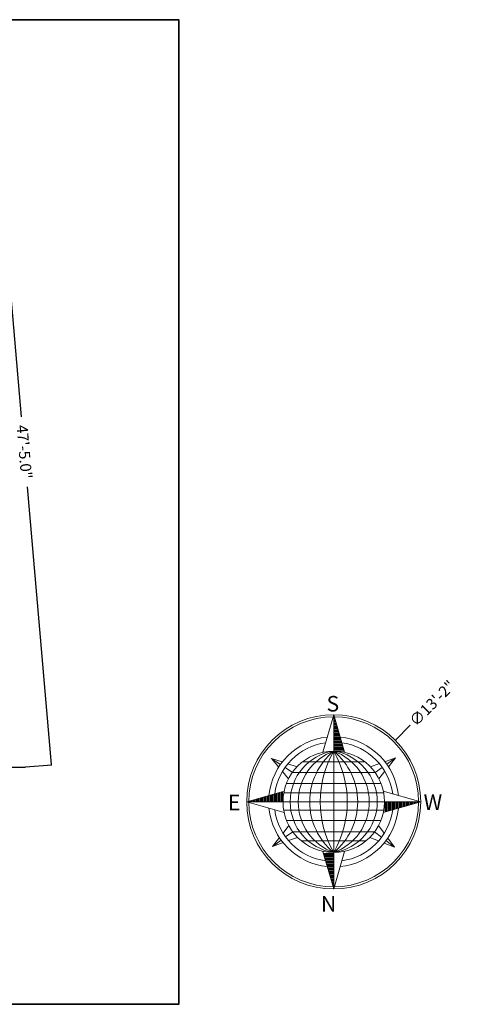
# Model space of a CAD drawing. Units: inches. Extents: x -269 to 4574, y -694 to 313.
# Tile 17 of 19: x 522 to 919, y -694 to 198. Entities that reach past the tile are written whole.
import ezdxf

# ---------------------------------------------------------------- set-up
doc = ezdxf.new("R2010")
doc.units = ezdxf.units.IN
doc.header["$MEASUREMENT"] = 0
for name, color, linetype, lineweight in [('A-ANNO-SYMB', 7, 'Continuous', 18), ('A-ANNO-SYMB-PATT', 7, 'Continuous', 13), ('BORDER', 7, 'Continuous', 35), ('C-PROP', 7, 'Continuous', 25), ('DIMENSION', 5, 'Continuous', 18)]:
    doc.layers.add(name, color=color, linetype=linetype, lineweight=lineweight)
doc.dimstyles.get("Standard").update_dxf_attribs({"dimtxt": 10, "dimasz": 0.18, "dimexe": 0.18, "dimexo": 0.0625, "dimgap": 0.09, "dimtad": 0, "dimdec": 1, "dimzin": 0, "dimdsep": 46, "dimlunit": 3, "dimtxsty": 'Standard', "dimcen": 0.09, "dimclrt": 7, "dimadec": 0, "dimazin": 0, "dimtfac": 1, "dimtdec": 1, "dimtofl": 0, "dimtmove": 0, "dimatfit": 3, "dimfxl": 1, "dimtolj": 1, "dimtzin": 0, "dimarcsym": 0})
pattern_1 = [(90, (-1638.3669, -937.0711), (-1, 0), [])]
pattern_2 = [(180, (-1638.3669, -937.0711), (-1e-16, -1), [])]

# ---------------------------------------------------------------- blocks, each defined once
blk = doc.blocks.new('*D35')
at = {"layer": 'Defpoints', "color": 0, "lineweight": 0, "transparency": 16777216}
for p in [(478.29, 88), (527.63, -478.86), (551.23, -476.8)]:
    blk.add_point(p, dxfattribs=at)
at = {"layer": 'DIMENSION', "color": 0, "lineweight": -2, "transparency": 16777216}
for p, q in [((478.36, 88.01), (502.07, 90.07)), ((501.91, 89.87), (523.81, -161.74)), ((551.21, -476.62), (529.31, -225.01)), ((527.69, -478.85), (551.41, -476.79))]:
    blk.add_line(p, q, dxfattribs=at)
at = {"layer": 'DIMENSION', "color": 0, "lineweight": 0, "transparency": 16777216}
for points in [[(501.94, 89.88), (501.88, 89.87), (501.89, 90.05)], [(551.24, -476.62), (551.18, -476.63), (551.23, -476.8)]]:
    blk.add_solid(points, dxfattribs=at)
at = {"layer": 'DIMENSION', "color": 0, "transparency": 16777216, "insert": (526.56, -193.38), "char_height": 10, "attachment_point": 5, "rotation": 274.97381}
blk.add_mtext('\\A1;47\'-5.0"', dxfattribs=at)
blk = doc.blocks.new('*D87')
at = {"layer": 'Defpoints', "color": 0, "lineweight": 0, "transparency": 16777216}
for p in [(862.88, -454.59), (751.27, -566.21)]:
    blk.add_point(p, dxfattribs=at)
at = {"layer": 'DIMENSION', "color": 0, "lineweight": -2, "transparency": 16777216}
for p, q in [((876.43, -441.04), (863, -454.47)), ((806.98, -510.4), (807.16, -510.4)), ((807.07, -510.49), (807.07, -510.31))]:
    blk.add_line(p, q, dxfattribs=at)
at = {"layer": 'DIMENSION', "color": 0, "lineweight": 0, "transparency": 16777216}
blk.add_solid([(862.98, -454.44), (863.03, -454.49), (862.88, -454.59)], dxfattribs=at)
at = {"layer": 'DIMENSION', "color": 7, "transparency": 16777216, "insert": (896.36, -421.11), "char_height": 10, "attachment_point": 5, "rotation": 45.00056}
blk.add_mtext('\\A1;∅13\'-2"', dxfattribs=at)

msp = doc.modelspace()

# ---------------------------------------------------------------- hatches: boundary and pattern name
at = {"layer": 'A-ANNO-SYMB-PATT'}
h = msp.add_hatch(dxfattribs=at)
h.set_pattern_fill('ANSI31', color=256, scale=8, angle=135, style=0)
h.set_pattern_definition(pattern_2)
h.paths.add_polyline_path([(807.07, -431.48), (807.07, -464.43), (816.51, -464.43)])
h = msp.add_hatch(dxfattribs=at)
h.set_pattern_fill('ANSI31', color=256, scale=8, angle=45, style=0)
h.set_pattern_definition(pattern_1)
h.paths.add_polyline_path([(728.15, -510.4), (761.1, -510.4), (761.1, -500.96)])
h = msp.add_hatch(dxfattribs=at)
h.set_pattern_fill('ANSI31', color=256, scale=8, angle=45, style=0)
h.set_pattern_definition(pattern_1)
h.paths.add_polyline_path([(885.99, -510.4), (853.04, -510.4), (853.04, -519.84)])
h = msp.add_hatch(dxfattribs=at)
h.set_pattern_fill('ANSI31', color=256, scale=8, angle=135, style=0)
h.set_pattern_definition(pattern_2)
h.paths.add_polyline_path([(807.07, -589.32), (807.07, -556.37), (797.63, -556.37)])

# ---------------------------------------------------------------- linework, layer by layer
at = {"layer": 'A-ANNO-SYMB'}
for p, q in [((807.07, -431.48), (797.34, -465.47)), ((807.07, -464.43), (807.07, -431.48)), ((807.07, -431.48), (816.81, -465.47)), ((758.76, -476.59), (750.48, -471.04)), ((750.58, -471.14), (757.19, -478.95)), ((750.58, -471.14), (760.44, -474.31)), ((807.07, -556.37), (807.07, -464.43)), ((863.05, -470.62), (853.49, -474.04)), ((855.16, -476.28), (863.05, -470.62)), ((863.05, -470.62), (856.73, -478.6)), ((769.56, -483.83), (762.91, -479.37)), ((765.53, -475.95), (773.85, -478.63)), ((778.77, -474.17), (835.37, -474.17)), ((848.51, -475.82), (840.38, -478.72)), ((844.6, -483.85), (851.1, -479.19)), ((760.59, -482.98), (766.12, -489.52)), ((769.59, -483.79), (844.56, -483.79)), ((853.43, -482.77), (848.05, -489.57)), ((764.19, -493.85), (849.96, -493.85)), ((728.15, -510.4), (762.15, -500.66)), ((761.85, -502.12), (852.29, -502.12)), ((885.99, -510.4), (852, -500.66)), ((761.1, -510.4), (728.15, -510.4)), ((728.15, -510.4), (762.15, -520.14)), ((761.1, -510.4), (853.04, -510.4)), ((885.99, -510.4), (852, -520.14)), ((853.04, -510.4), (885.99, -510.4)), ((761.71, -517.85), (852.43, -517.85)), ((761.11, -538.68), (766.44, -531.91)), ((764.39, -527.47), (849.75, -527.47)), ((852.91, -538.88), (847.73, -531.84)), ((751.55, -550.82), (757.83, -542.85)), ((769.97, -537.54), (763.48, -542.22)), ((766.13, -545.56), (774.29, -542.62)), ((769.96, -537.53), (844.18, -537.53)), ((847.81, -545.8), (839.85, -542.63)), ((844.16, -537.56), (850.49, -542.45)), ((862.21, -551.54), (856.08, -543.19)), ((759.42, -545.14), (751.55, -550.82)), ((751.55, -550.82), (761.13, -547.37)), ((777.75, -545.8), (836.39, -545.8)), ((862.21, -551.54), (852.7, -547.75)), ((854.45, -545.51), (862.33, -551.6)), ((807.07, -589.32), (797.34, -555.32)), ((807.07, -589.32), (816.81, -555.32)), ((807.07, -556.37), (807.07, -589.32))]:
    msp.add_line(p, q, dxfattribs=at)
for radius in [78.92, 76.97, 45.97]:
    msp.add_circle((807.07, -510.4), radius, dxfattribs=at)
for centre, radius, start, end in [((807.07, -510.4), 58.97, 95.64079, 174.35921), ((807.07, -510.4), 58.97, 5.64079, 84.35921), ((807.07, -510.4), 53.97, 97.76092, 172.23908), ((807.07, -510.4), 53.97, 7.76092, 82.23908), ((814.06, -510.4), 46.5, 98.64449, 261.35551), ((823.77, -510.4), 48.91, 109.96876, 250.03124), ((844.78, -510.4), 59.46, 129.3656, 230.6344), ((887.18, -510.4), 92.36, 150.15267, 209.84733), ((887.18, -510.4), 92.36, 150.15267, 209.84733), ((726.96, -510.4), 92.36, 330.15267, 29.84733), ((769.36, -510.4), 59.46, 309.3656, 50.6344), ((790.37, -510.4), 48.91, 289.96876, 70.03124), ((800.08, -510.4), 46.5, 278.64449, 81.35551), ((807.07, -510.4), 58.97, 185.64079, 264.35921), ((807.07, -510.4), 58.97, 275.64079, 354.35921), ((807.07, -510.4), 53.97, 187.76092, 262.23908), ((807.07, -510.4), 53.97, 277.76092, 352.23908)]:
    msp.add_arc(centre, radius, start, end, dxfattribs=at)
at = {"layer": 'BORDER'}
msp.add_lwpolyline([(-268.51, 198.09), (666.62, 198.09), (666.62, -693.82), (-268.51, -693.82)], close=True, dxfattribs=at)
at = {"layer": 'C-PROP'}
msp.add_line((-68.45, -480.67), (527.63, -478.86), dxfattribs=at)

# ---------------------------------------------------------------- texts
at = {"layer": 'A-ANNO-SYMB'}
for s, p in [('S', (800.59, -428.55)), ('E', (711.18, -517.97)), ('W', (888.59, -517.77)), ('N', (795.53, -609.89))]:
    msp.add_text(s, height=14.04, dxfattribs=at).set_placement(p)

# ---------------------------------------------------------------- dimensions: what is measured, and where the dimension line sits
at = {"layer": 'DIMENSION'}
dim = msp.add_aligned_dim(p1=(478.29, 88), p2=(527.63, -478.86), distance=23.69, dimstyle='Standard', override={"dimclrd": 0, "dimclre": 0, "dimclrt": 0}, dxfattribs=at)
dim.commit()
dim.dimension.update_dxf_attribs({"geometry": '*D35', "text_midpoint": (526.56, -193.38)})
dim = msp.add_diameter_dim_2p(p1=(751.27, -566.21), p2=(862.88, -454.59), dimstyle='Standard', override={"dimdec": 1, "dimlfac": 1, "dimrnd": 0, "dimzin": 1, "dimdsep": 46, "dimlunit": 4, "dimfrac": 2}, dxfattribs=at)
dim.commit()
dim.dimension.update_dxf_attribs({"geometry": '*D87', "text_midpoint": (896.36, -421.11), "dimtype": 163})

doc.saveas('drawing.dxf')
